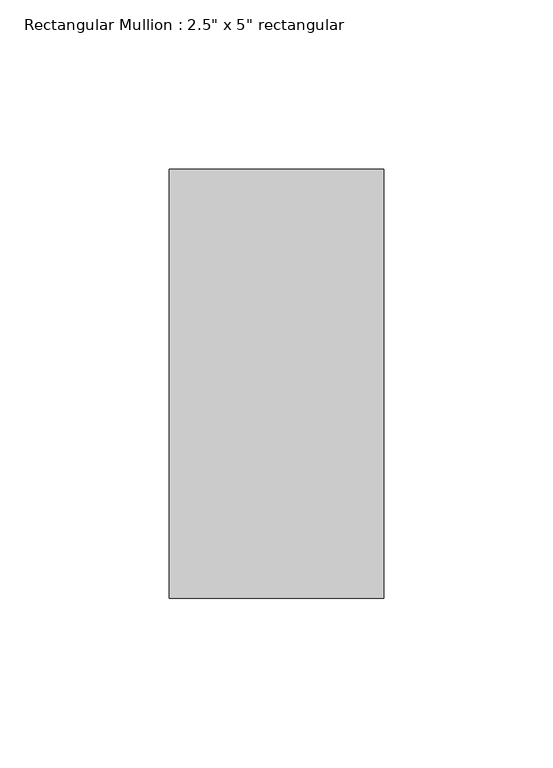
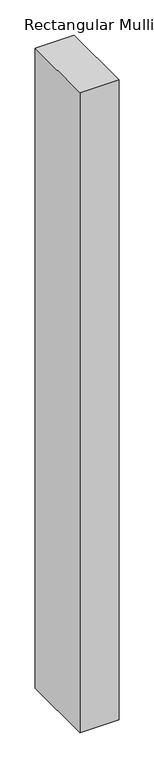
"""IFC4 building model written with IfcOpenShell, lengths in millimetres: member geometry."""

from ifc_helpers import new_model, si_unit, frame, origin, place, context, project, spatial, polyline, outline, extrude, source, transform, mapped, element, save


def member_d69c7880(model_context):
    return source(origin(), model_context, "Body", "SweptSolid", [
        extrude(outline(polyline([(0.0, 63.5), (0.0, -63.5), (-63.5, -63.5), (-63.5, 63.5), (0.0, 63.5)])), frame((0.0, 0.0, -1104.9000002), z_axis=(0.0, 0.0, 1.0), x_axis=(1.0, 0.0, 0.0)), (0.0, 0.0, 1.0), 1104.9000002),
    ])


if __name__ == "__main__":
    model = new_model("IFC4")
    model_context = context("Model", 3, world=origin())
    ifc_project = project(units=[si_unit("LENGTHUNIT", "METRE", prefix="MILLI")], contexts=[model_context])
    site = spatial("IfcSite", under=ifc_project)
    building = spatial("IfcBuilding", under=site)
    placement = place(None, origin())
    member_shape = member_d69c7880(model_context)
    element("IfcMember", 1, ObjectType="Rectangular Mullion : 2.5\" x 5\" rectangular", at=placement, inside=building, context=model_context, shape_type="MappedRepresentation", body=[
        mapped(member_shape, transform((0.0, 0.0, 0.0), x_axis=(1.0, 0.0, 0.0), y_axis=(0.0, 1.0, 0.0), z_axis=(0.0, 0.0, 1.0))),
    ])
    save(model, "model.ifc")

# Revit data of these elements
# Type "Rectangular Mullion : 2.5\" x 5\" rectangular"
#   built-in parameter 1007304 = 0.416667 (stored number, unit not read)
#   built-in parameter 1007301 = 0.104167 (stored number, unit not read)
#   built-in parameter 1007300 = 0.104167 (stored number, unit not read)
# Element 1 (IfcMember, "Rectangular Mullion : 2.5\" x 5\" rectangular")
#   Materials on its faces: "BLACK COLOUR"
# Materials
#   "BLACK COLOUR": class "Generic", colour RGB 120 120 120, transparency 0, Cost = 0
